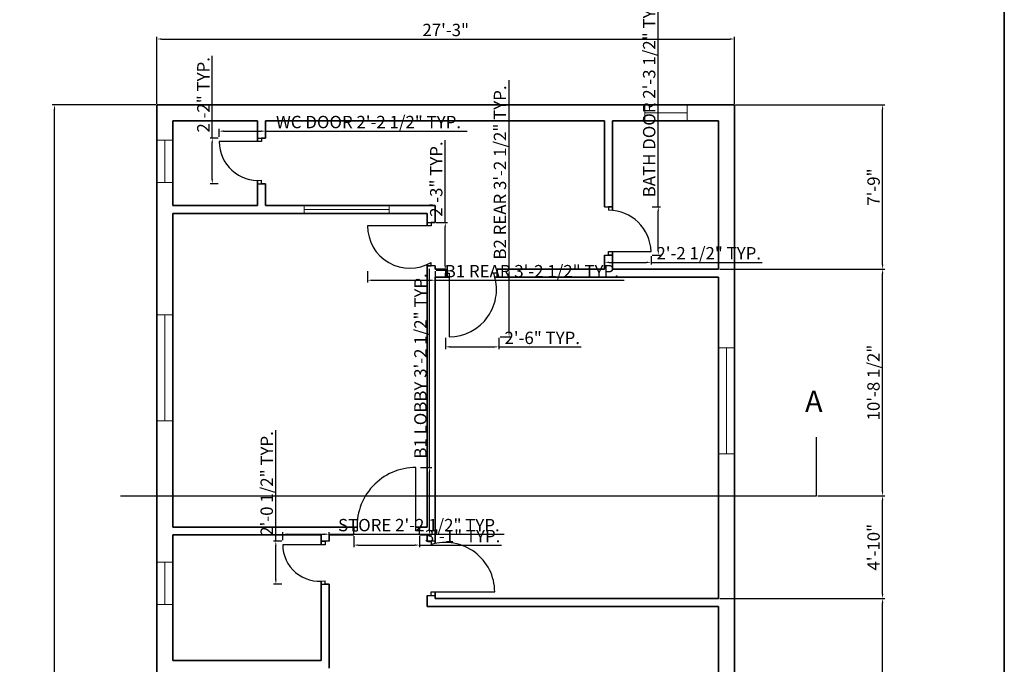
# Model space of a CAD drawing. Units: inches. Extents: x 1863 to 2938, y 1238 to 2492.
# Tile 11 of 12: x 2381 to 2938, y 1760 to 2125. Entities that reach past the tile are written whole.
import ezdxf

# ---------------------------------------------------------------- set-up
doc = ezdxf.new("R2010")
doc.units = ezdxf.units.IN
for name, color, linetype, lineweight in [('A-ANNO-DIMS', 2, 'Continuous', 18), ('A-ANNO-SYMB', 7, 'Continuous', 25), ('A-ANNO-TTLB', 7, 'Continuous', 35), ('A-DOOR', 3, 'Continuous', 25), ('A-GLAZ', 4, 'Continuous', 18), ('A-WALL', 7, 'Continuous', 35)]:
    doc.layers.add(name, color=color, linetype=linetype, lineweight=lineweight)
doc.styles.get("Standard").update_dxf_attribs({"font": 'arial.ttf'})
doc.dimstyles.new('ISO-25', dxfattribs={"dimtxt": 7, "dimasz": 2.5, "dimexe": 1.25, "dimexo": 0.625, "dimtad": 1, "dimdec": 0, "dimlunit": 3, "dimtxsty": 'Standard', "dimcen": 2.5, "dimadec": 0, "dimazin": 0, "dimtfac": 1, "dimtdec": 0, "dimtmove": 0, "dimatfit": 3, "dimfxl": 1, "dimarcsym": 0})

# ---------------------------------------------------------------- blocks, each defined once
blk = doc.blocks.new('DOOR-24-TOILET')
for p, q in [((24, 23.86), (0, 23.86)), ((21.75, 25.86), (26.25, 25.86)), ((26.25, 25.86), (24, 25.86)), ((24, 25.86), (24, 23.86)), ((21.75, 0), (26.25, 0)), ((24, 0), (24, 2)), ((26.25, 0), (24, 0))]:
    blk.add_line(p, q)
blk.add_arc((21.96, 23.86), 21.96, 180, 275.3383)
blk = doc.blocks.new('DOOR-36-BED1-REAR')
for p, q in [((36, 23.94), (0, 23.94)), ((33.75, 25.94), (38.25, 25.94)), ((38.25, 25.94), (36, 25.94)), ((36, 25.94), (36, 23.94)), ((38.25, 1.26), (33.75, 1.26)), ((33.75, 1.26), (36, 1.26)), ((36, 1.26), (36, 3.26))]:
    blk.add_line(p, q)
blk.add_arc((23.94, 23.94), 23.94, 180, 300.2375)
blk = doc.blocks.new('DOOR-24-BATH')
for p, q in [((0, 27.38), (4.5, 27.38)), ((4.5, 27.38), (2.25, 27.38)), ((2.25, 27.38), (2.25, 25.38)), ((0, 0), (4.5, 0)), ((2.25, 0), (2.25, 2)), ((2.25, 2), (26.25, 2)), ((4.5, 0), (2.25, 0))]:
    blk.add_line(p, q)
blk.add_arc((2.25, 1.37), 24.01, 1.5021, 90)
blk = doc.blocks.new('DOOR-36-BED2-REAR')
for p, q in [((0, 38.25), (0, 33.75)), ((0, 33.75), (0, 36)), ((0, 36), (2, 36)), ((2, 36), (2, 0)), ((29.25, 36), (27.25, 36)), ((29.25, 38.25), (29.25, 33.75)), ((29.25, 33.75), (29.25, 36))]:
    blk.add_line(p, q)
blk.add_arc((2, 26.86), 26.86, 270, 19.9084)
blk = doc.blocks.new('DOOR-36-BED2-LOBBY')
for p, q in [((0, 30.86), (4.5, 30.86)), ((2.25, 30.86), (2.25, 28.86)), ((0, 0), (4.5, 0)), ((2.25, 0), (2.25, 2)), ((2.25, 2), (38.25, 2))]:
    blk.add_line(p, q)
blk.add_arc((10.23, 2), 28.02, 0, 106.5507)
blk = doc.blocks.new('DOOR-24-STORE')
for p, q in [((24, 22.39), (0, 22.39)), ((26.25, 24.39), (21.75, 24.39)), ((21.75, 24.39), (24, 24.39)), ((24, 24.39), (24, 22.39)), ((24, 0), (24, 2)), ((21.75, 0), (26.25, 0)), ((26.25, 0), (24, 0))]:
    blk.add_line(p, q)
blk.add_arc((20.66, 22.39), 20.66, 180, 279.3111)
blk = doc.blocks.new('DOOR-36-BED1-LOBBY')
for p, q in [((35.21, 2.25), (35.21, 38.25)), ((0, 0), (0, 4.5)), ((0, 4.5), (0, 2.25)), ((0, 2.25), (2, 2.25)), ((37.21, 2.25), (35.21, 2.25)), ((37.21, 0), (37.21, 4.5)), ((37.21, 4.5), (37.21, 2.25))]:
    blk.add_line(p, q)
blk.add_arc((35.21, 4.93), 33.32, 90, 184.6101)
blk = doc.blocks.new('WIN-24')
for p, q in [((0, 24), (9, 24)), ((9, 24), (4.5, 24)), ((4.5, 24), (4.5, 0)), ((4.5, 0), (0, 0)), ((0, 0), (9, 0))]:
    blk.add_line(p, q)
blk = doc.blocks.new('WIN-48')
for p, q in [((0, 4.5), (0, 0)), ((0, 0), (0, 2.25)), ((0, 2.25), (48, 2.25)), ((48, 2.25), (48, 4.5)), ((48, 4.5), (48, 0))]:
    blk.add_line(p, q)
blk = doc.blocks.new('WIN-60')
for p, q in [((0, 60), (9, 60)), ((9, 60), (4.5, 60)), ((4.5, 60), (4.5, 0)), ((4.5, 0), (0, 0)), ((0, 0), (9, 0))]:
    blk.add_line(p, q)
blk = doc.blocks.new('WIN-24-STORE')
for p, q in [((0, 24), (9, 24)), ((9, 24), (4.5, 24)), ((4.5, 24), (4.5, 0)), ((9, 0), (0, 0)), ((4.5, 0), (9, 0))]:
    blk.add_line(p, q)
blk = doc.blocks.new('*D40')
at = {"layer": 'A-ANNO-DIMS', "color": 0, "lineweight": -2, "transparency": 16777216}
for p, q in [((2493.88, 2058.42), (2493.88, 2062.98)), ((2520.13, 2058.42), (2520.13, 2062.98)), ((2496.38, 2061.73), (2517.63, 2061.73)), ((2520.13, 2061.73), (2634.21, 2061.73))]:
    blk.add_line(p, q, dxfattribs=at)
at = {"layer": 'A-ANNO-DIMS', "color": 0, "transparency": 16777216}
for points in [[(2496.38, 2062.15), (2496.38, 2061.31), (2493.88, 2061.73)], [(2517.63, 2062.15), (2517.63, 2061.31), (2520.13, 2061.73)]]:
    blk.add_solid(points, dxfattribs=at)
at = {"layer": 'Defpoints', "color": 0, "transparency": 16777216}
for p in [(2493.88, 2057.79), (2520.13, 2061.73), (2520.13, 2057.79)]:
    blk.add_point(p, dxfattribs=at)
at = {"layer": 'A-ANNO-DIMS', "color": 0, "transparency": 16777216, "insert": (2578.42, 2065.98), "char_height": 7, "attachment_point": 5}
blk.add_mtext('WC DOOR 2\'-2 1/2" TYP.', dxfattribs=at)
blk = doc.blocks.new('*D41')
at = {"layer": 'A-ANNO-DIMS', "color": 0, "lineweight": -2, "transparency": 16777216}
for p, q in [((2489.94, 2057.79), (2489.94, 2104.33)), ((2493.26, 2057.79), (2488.69, 2057.79)), ((2489.94, 2034.43), (2489.94, 2055.29)), ((2493.26, 2031.93), (2488.69, 2031.93))]:
    blk.add_line(p, q, dxfattribs=at)
at = {"layer": 'A-ANNO-DIMS', "color": 0, "transparency": 16777216}
for points in [[(2489.53, 2055.29), (2490.36, 2055.29), (2489.94, 2057.79)], [(2489.53, 2034.43), (2490.36, 2034.43), (2489.94, 2031.93)]]:
    blk.add_solid(points, dxfattribs=at)
at = {"layer": 'Defpoints', "color": 0, "transparency": 16777216}
for p in [(2489.94, 2057.79), (2493.88, 2057.79), (2493.88, 2031.93)]:
    blk.add_point(p, dxfattribs=at)
at = {"layer": 'A-ANNO-DIMS', "color": 0, "transparency": 16777216, "insert": (2485.8, 2082.31), "char_height": 7, "attachment_point": 5, "rotation": 90}
blk.add_mtext('2\'-2" TYP.', dxfattribs=at)
blk = doc.blocks.new('*D42')
at = {"layer": 'A-ANNO-DIMS', "color": 0, "lineweight": -2, "transparency": 16777216}
for p, q in [((2577.88, 1982.4), (2577.88, 1976.04)), ((2616.13, 1982.4), (2616.13, 1976.04)), ((2580.38, 1977.29), (2613.63, 1977.29)), ((2616.13, 1977.29), (2723.11, 1977.29))]:
    blk.add_line(p, q, dxfattribs=at)
at = {"layer": 'A-ANNO-DIMS', "color": 0, "transparency": 16777216}
for points in [[(2580.38, 1977.7), (2580.38, 1976.87), (2577.88, 1977.29)], [(2613.63, 1977.7), (2613.63, 1976.87), (2616.13, 1977.29)]]:
    blk.add_solid(points, dxfattribs=at)
at = {"layer": 'Defpoints', "color": 0, "transparency": 16777216}
for p in [(2577.88, 1983.02), (2616.13, 1983.02), (2616.13, 1977.29)]:
    blk.add_point(p, dxfattribs=at)
at = {"layer": 'A-ANNO-DIMS', "color": 0, "transparency": 16777216, "insert": (2670.87, 1981.53), "char_height": 7, "attachment_point": 5}
blk.add_mtext('B1 REAR 3\'-2 1/2" TYP.', dxfattribs=at)
blk = doc.blocks.new('*D43')
at = {"layer": 'A-ANNO-DIMS', "color": 0, "lineweight": -2, "transparency": 16777216}
for p, q in [((2621.87, 2010.05), (2621.87, 2056.59)), ((2616.76, 2010.05), (2623.12, 2010.05)), ((2621.87, 1985.52), (2621.87, 2007.55)), ((2616.76, 1983.02), (2623.12, 1983.02))]:
    blk.add_line(p, q, dxfattribs=at)
at = {"layer": 'A-ANNO-DIMS', "color": 0, "transparency": 16777216}
for points in [[(2621.45, 2007.55), (2622.29, 2007.55), (2621.87, 2010.05)], [(2621.45, 1985.52), (2622.29, 1985.52), (2621.87, 1983.02)]]:
    blk.add_solid(points, dxfattribs=at)
at = {"layer": 'Defpoints', "color": 0, "transparency": 16777216}
for p in [(2616.13, 2010.05), (2621.87, 2010.05), (2616.13, 1983.02)]:
    blk.add_point(p, dxfattribs=at)
at = {"layer": 'A-ANNO-DIMS', "color": 0, "transparency": 16777216, "insert": (2617.67, 2034.57), "char_height": 7, "attachment_point": 5, "rotation": 90}
blk.add_mtext('2\'-3" TYP.', dxfattribs=at)
blk = doc.blocks.new('*D44')
at = {"layer": 'A-ANNO-DIMS', "color": 0, "lineweight": -2, "transparency": 16777216}
for p, q in [((2742.49, 2018.92), (2742.49, 2142.19)), ((2739.01, 2018.92), (2743.74, 2018.92)), ((2742.49, 1994.04), (2742.49, 2016.42)), ((2739.01, 1991.54), (2743.74, 1991.54))]:
    blk.add_line(p, q, dxfattribs=at)
at = {"layer": 'A-ANNO-DIMS', "color": 0, "transparency": 16777216}
for points in [[(2742.07, 2016.42), (2742.91, 2016.42), (2742.49, 2018.92)], [(2742.07, 1994.04), (2742.91, 1994.04), (2742.49, 1991.54)]]:
    blk.add_solid(points, dxfattribs=at)
at = {"layer": 'Defpoints', "color": 0, "transparency": 16777216}
for p in [(2738.38, 2018.92), (2742.49, 2018.92), (2738.38, 1991.54)]:
    blk.add_point(p, dxfattribs=at)
at = {"layer": 'A-ANNO-DIMS', "color": 0, "transparency": 16777216, "insert": (2738.24, 2081.8), "char_height": 7, "attachment_point": 5, "rotation": 90}
blk.add_mtext('BATH DOOR 2\'-3 1/2" TYP.', dxfattribs=at)
blk = doc.blocks.new('*D45')
at = {"layer": 'A-ANNO-DIMS', "color": 0, "lineweight": -2, "transparency": 16777216}
for p, q in [((2712.13, 1990.91), (2712.13, 1986.18)), ((2738.38, 1990.91), (2738.38, 1986.18)), ((2714.63, 1987.43), (2735.88, 1987.43)), ((2738.38, 1987.43), (2801.23, 1987.43))]:
    blk.add_line(p, q, dxfattribs=at)
at = {"layer": 'A-ANNO-DIMS', "color": 0, "transparency": 16777216}
for points in [[(2714.63, 1987.85), (2714.63, 1987.01), (2712.13, 1987.43)], [(2735.88, 1987.85), (2735.88, 1987.01), (2738.38, 1987.43)]]:
    blk.add_solid(points, dxfattribs=at)
at = {"layer": 'Defpoints', "color": 0, "transparency": 16777216}
for p in [(2712.13, 1991.54), (2738.38, 1991.54), (2738.38, 1987.43)]:
    blk.add_point(p, dxfattribs=at)
at = {"layer": 'A-ANNO-DIMS', "color": 0, "transparency": 16777216, "insert": (2771.06, 1991.68), "char_height": 7, "attachment_point": 5}
blk.add_mtext('2\'-2 1/2" TYP.', dxfattribs=at)
blk = doc.blocks.new('*D46')
at = {"layer": 'A-ANNO-DIMS', "color": 0, "lineweight": -2, "transparency": 16777216}
for p, q in [((2658.01, 1983.56), (2658.01, 2090.55)), ((2652.89, 1983.56), (2659.26, 1983.56)), ((2658.01, 1947.81), (2658.01, 1981.06)), ((2652.89, 1945.31), (2659.26, 1945.31))]:
    blk.add_line(p, q, dxfattribs=at)
at = {"layer": 'A-ANNO-DIMS', "color": 0, "transparency": 16777216}
for points in [[(2657.59, 1981.06), (2658.42, 1981.06), (2658.01, 1983.56)], [(2657.59, 1947.81), (2658.42, 1947.81), (2658.01, 1945.31)]]:
    blk.add_solid(points, dxfattribs=at)
at = {"layer": 'Defpoints', "color": 0, "transparency": 16777216}
for p in [(2652.27, 1983.56), (2658.01, 1983.56), (2652.27, 1945.31)]:
    blk.add_point(p, dxfattribs=at)
at = {"layer": 'A-ANNO-DIMS', "color": 0, "transparency": 16777216, "insert": (2653.76, 2038.3), "char_height": 7, "attachment_point": 5, "rotation": 90}
blk.add_mtext('B2 REAR 3\'-2 1/2" TYP.', dxfattribs=at)
blk = doc.blocks.new('*D47')
at = {"layer": 'A-ANNO-DIMS', "color": 0, "lineweight": -2, "transparency": 16777216}
for p, q in [((2622.04, 1944.69), (2622.04, 1938.32)), ((2652.27, 1944.69), (2652.27, 1938.32)), ((2624.54, 1939.57), (2649.77, 1939.57)), ((2652.27, 1939.57), (2698.81, 1939.57))]:
    blk.add_line(p, q, dxfattribs=at)
at = {"layer": 'A-ANNO-DIMS', "color": 0, "transparency": 16777216}
for points in [[(2624.54, 1939.99), (2624.54, 1939.16), (2622.04, 1939.57)], [(2649.77, 1939.99), (2649.77, 1939.16), (2652.27, 1939.57)]]:
    blk.add_solid(points, dxfattribs=at)
at = {"layer": 'Defpoints', "color": 0, "transparency": 16777216}
for p in [(2622.04, 1945.31), (2652.27, 1945.31), (2652.27, 1939.57)]:
    blk.add_point(p, dxfattribs=at)
at = {"layer": 'A-ANNO-DIMS', "color": 0, "transparency": 16777216, "insert": (2676.79, 1943.77), "char_height": 7, "attachment_point": 5}
blk.add_mtext('2\'-6" TYP.', dxfattribs=at)
blk = doc.blocks.new('*D50')
at = {"layer": 'A-ANNO-DIMS', "color": 0, "lineweight": -2, "transparency": 16777216}
for p, q in [((2529.88, 1830.17), (2529.88, 1834.73)), ((2556.13, 1830.17), (2556.13, 1834.73)), ((2532.38, 1833.48), (2553.63, 1833.48)), ((2556.13, 1833.48), (2655.23, 1833.48))]:
    blk.add_line(p, q, dxfattribs=at)
at = {"layer": 'A-ANNO-DIMS', "color": 0, "transparency": 16777216}
for points in [[(2532.38, 1833.9), (2532.38, 1833.06), (2529.88, 1833.48)], [(2553.63, 1833.9), (2553.63, 1833.06), (2556.13, 1833.48)]]:
    blk.add_solid(points, dxfattribs=at)
at = {"layer": 'Defpoints', "color": 0, "transparency": 16777216}
for p in [(2529.88, 1829.54), (2556.13, 1833.48), (2556.13, 1829.54)]:
    blk.add_point(p, dxfattribs=at)
at = {"layer": 'A-ANNO-DIMS', "color": 0, "transparency": 16777216, "insert": (2606.93, 1837.73), "char_height": 7, "attachment_point": 5}
blk.add_mtext('STORE 2\'-2 1/2" TYP.', dxfattribs=at)
blk = doc.blocks.new('*D51')
at = {"layer": 'A-ANNO-DIMS', "color": 0, "lineweight": -2, "transparency": 16777216}
for p, q in [((2525.94, 1829.54), (2525.94, 1892.39)), ((2529.26, 1829.54), (2524.69, 1829.54)), ((2525.94, 1807.66), (2525.94, 1827.04)), ((2529.26, 1805.16), (2524.69, 1805.16))]:
    blk.add_line(p, q, dxfattribs=at)
at = {"layer": 'A-ANNO-DIMS', "color": 0, "transparency": 16777216}
for points in [[(2525.53, 1827.04), (2526.36, 1827.04), (2525.94, 1829.54)], [(2525.53, 1807.66), (2526.36, 1807.66), (2525.94, 1805.16)]]:
    blk.add_solid(points, dxfattribs=at)
at = {"layer": 'Defpoints', "color": 0, "transparency": 16777216}
for p in [(2525.94, 1829.54), (2529.88, 1829.54), (2529.88, 1805.16)]:
    blk.add_point(p, dxfattribs=at)
at = {"layer": 'A-ANNO-DIMS', "color": 0, "transparency": 16777216, "insert": (2521.7, 1862.22), "char_height": 7, "attachment_point": 5, "rotation": 90}
blk.add_mtext('2\'-0 1/2" TYP.', dxfattribs=at)
blk = doc.blocks.new('*D52')
at = {"layer": 'A-ANNO-DIMS', "color": 0, "lineweight": -2, "transparency": 16777216}
for p, q in [((2612.98, 1871.31), (2612.98, 1983.74)), ((2607.87, 1871.31), (2614.23, 1871.31)), ((2612.98, 1835.56), (2612.98, 1868.81)), ((2607.87, 1833.06), (2614.23, 1833.06))]:
    blk.add_line(p, q, dxfattribs=at)
at = {"layer": 'A-ANNO-DIMS', "color": 0, "transparency": 16777216}
for points in [[(2612.56, 1868.81), (2613.4, 1868.81), (2612.98, 1871.31)], [(2612.56, 1835.56), (2613.4, 1835.56), (2612.98, 1833.06)]]:
    blk.add_solid(points, dxfattribs=at)
at = {"layer": 'Defpoints', "color": 0, "transparency": 16777216}
for p in [(2607.24, 1871.31), (2612.98, 1871.31), (2607.24, 1833.06)]:
    blk.add_point(p, dxfattribs=at)
at = {"layer": 'A-ANNO-DIMS', "color": 0, "transparency": 16777216, "insert": (2608.73, 1928.78), "char_height": 7, "attachment_point": 5, "rotation": 90}
blk.add_mtext('B1 LOBBY 3\'-2 1/2" TYP.', dxfattribs=at)
blk = doc.blocks.new('*D53')
at = {"layer": 'A-ANNO-DIMS', "color": 0, "lineweight": -2, "transparency": 16777216}
for p, q in [((2570.03, 1832.44), (2570.03, 1826.07)), ((2607.24, 1832.44), (2607.24, 1826.07)), ((2572.53, 1827.32), (2604.74, 1827.32)), ((2607.24, 1827.32), (2653.66, 1827.32))]:
    blk.add_line(p, q, dxfattribs=at)
at = {"layer": 'A-ANNO-DIMS', "color": 0, "transparency": 16777216}
for points in [[(2572.53, 1827.74), (2572.53, 1826.91), (2570.03, 1827.32)], [(2604.74, 1827.74), (2604.74, 1826.91), (2607.24, 1827.32)]]:
    blk.add_solid(points, dxfattribs=at)
at = {"layer": 'Defpoints', "color": 0, "transparency": 16777216}
for p in [(2570.03, 1833.06), (2607.24, 1833.06), (2607.24, 1827.32)]:
    blk.add_point(p, dxfattribs=at)
at = {"layer": 'A-ANNO-DIMS', "color": 0, "transparency": 16777216, "insert": (2631.7, 1831.53), "char_height": 7, "attachment_point": 5}
blk.add_mtext('3\'-1" TYP.', dxfattribs=at)
blk = doc.blocks.new('*D64')
at = {"layer": 'A-ANNO-DIMS', "color": 0, "lineweight": -2, "transparency": 16777216}
for p, q in [((2458.63, 2077.19), (2458.63, 2115.16)), ((2461.13, 2113.91), (2783.13, 2113.91)), ((2785.63, 2077.19), (2785.63, 2115.16))]:
    blk.add_line(p, q, dxfattribs=at)
at = {"layer": 'A-ANNO-DIMS', "color": 0, "transparency": 16777216}
for points in [[(2461.13, 2114.33), (2461.13, 2113.5), (2458.63, 2113.91)], [(2783.13, 2114.33), (2783.13, 2113.5), (2785.63, 2113.91)]]:
    blk.add_solid(points, dxfattribs=at)
at = {"layer": 'Defpoints', "color": 0, "transparency": 16777216}
for p in [(2785.63, 2113.91), (2458.63, 2076.56), (2785.63, 2076.56)]:
    blk.add_point(p, dxfattribs=at)
at = {"layer": 'A-ANNO-DIMS', "color": 0, "transparency": 16777216, "insert": (2622.13, 2118.11), "char_height": 7, "attachment_point": 5}
blk.add_mtext('27\'-3"', dxfattribs=at)
blk = doc.blocks.new('*D65')
at = {"layer": 'A-ANNO-DIMS', "color": 0, "lineweight": -2, "transparency": 16777216}
for p, q in [((2458.01, 2076.56), (2399.39, 2076.56)), ((2400.64, 1342.06), (2400.64, 2074.06)), ((2458.01, 1339.56), (2399.39, 1339.56))]:
    blk.add_line(p, q, dxfattribs=at)
at = {"layer": 'A-ANNO-DIMS', "color": 0, "transparency": 16777216}
for points in [[(2400.22, 2074.06), (2401.06, 2074.06), (2400.64, 2076.56)], [(2400.22, 1342.06), (2401.06, 1342.06), (2400.64, 1339.56)]]:
    blk.add_solid(points, dxfattribs=at)
at = {"layer": 'Defpoints', "color": 0, "transparency": 16777216}
for p in [(2400.64, 2076.56), (2458.63, 2076.56), (2458.63, 1339.56)]:
    blk.add_point(p, dxfattribs=at)
at = {"layer": 'A-ANNO-DIMS', "color": 0, "transparency": 16777216, "insert": (2396.44, 1708.06), "char_height": 7, "attachment_point": 5, "rotation": 90}
blk.add_mtext('61\'-5"', dxfattribs=at)
blk = doc.blocks.new('*D67')
at = {"layer": 'A-ANNO-DIMS', "color": 0, "lineweight": -2, "transparency": 16777216}
for p, q in [((2777.26, 1797.06), (2870.74, 1797.06)), ((2869.49, 1579.06), (2869.49, 1794.56)), ((2777.26, 1576.56), (2870.74, 1576.56))]:
    blk.add_line(p, q, dxfattribs=at)
at = {"layer": 'A-ANNO-DIMS', "color": 0, "transparency": 16777216}
for points in [[(2869.07, 1794.56), (2869.91, 1794.56), (2869.49, 1797.06)], [(2869.07, 1579.06), (2869.91, 1579.06), (2869.49, 1576.56)]]:
    blk.add_solid(points, dxfattribs=at)
at = {"layer": 'Defpoints', "color": 0, "transparency": 16777216}
for p in [(2776.63, 1797.06), (2869.49, 1797.06), (2776.63, 1576.56)]:
    blk.add_point(p, dxfattribs=at)
at = {"layer": 'A-ANNO-DIMS', "color": 0, "transparency": 16777216, "insert": (2865.25, 1686.81), "char_height": 7, "attachment_point": 5, "rotation": 90}
blk.add_mtext('18\'-4 1/2"', dxfattribs=at)
blk = doc.blocks.new('*D68')
at = {"layer": 'A-ANNO-DIMS', "color": 0, "lineweight": -2, "transparency": 16777216}
for p, q in [((2832.77, 1855.17), (2870.74, 1855.17)), ((2869.49, 1799.56), (2869.49, 1852.67)), ((2777.26, 1797.06), (2870.74, 1797.06))]:
    blk.add_line(p, q, dxfattribs=at)
at = {"layer": 'A-ANNO-DIMS', "color": 0, "transparency": 16777216}
for points in [[(2869.07, 1852.67), (2869.91, 1852.67), (2869.49, 1855.17)], [(2869.07, 1799.56), (2869.91, 1799.56), (2869.49, 1797.06)]]:
    blk.add_solid(points, dxfattribs=at)
at = {"layer": 'Defpoints', "color": 0, "transparency": 16777216}
for p in [(2832.14, 1855.17), (2869.49, 1855.17), (2776.63, 1797.06)]:
    blk.add_point(p, dxfattribs=at)
at = {"layer": 'A-ANNO-DIMS', "color": 0, "transparency": 16777216, "insert": (2865.29, 1826.12), "char_height": 7, "attachment_point": 5, "rotation": 90}
blk.add_mtext('4\'-10"', dxfattribs=at)
blk = doc.blocks.new('*D69')
at = {"layer": 'A-ANNO-DIMS', "color": 0, "lineweight": -2, "transparency": 16777216}
for p, q in [((2777.26, 1983.56), (2870.74, 1983.56)), ((2869.49, 1857.67), (2869.49, 1981.06)), ((2832.77, 1855.17), (2870.74, 1855.17))]:
    blk.add_line(p, q, dxfattribs=at)
at = {"layer": 'A-ANNO-DIMS', "color": 0, "transparency": 16777216}
for points in [[(2869.07, 1981.06), (2869.91, 1981.06), (2869.49, 1983.56)], [(2869.07, 1857.67), (2869.91, 1857.67), (2869.49, 1855.17)]]:
    blk.add_solid(points, dxfattribs=at)
at = {"layer": 'Defpoints', "color": 0, "transparency": 16777216}
for p in [(2776.63, 1983.56), (2869.49, 1983.56), (2832.14, 1855.17)]:
    blk.add_point(p, dxfattribs=at)
at = {"layer": 'A-ANNO-DIMS', "color": 0, "transparency": 16777216, "insert": (2865.25, 1919.37), "char_height": 7, "attachment_point": 5, "rotation": 90}
blk.add_mtext('10\'-8 1/2"', dxfattribs=at)
blk = doc.blocks.new('*D70')
at = {"layer": 'A-ANNO-DIMS', "color": 0, "lineweight": -2, "transparency": 16777216}
for p, q in [((2786.26, 2076.56), (2870.74, 2076.56)), ((2869.49, 1986.06), (2869.49, 2074.06)), ((2777.26, 1983.56), (2870.74, 1983.56))]:
    blk.add_line(p, q, dxfattribs=at)
at = {"layer": 'A-ANNO-DIMS', "color": 0, "transparency": 16777216}
for points in [[(2869.07, 2074.06), (2869.91, 2074.06), (2869.49, 2076.56)], [(2869.07, 1986.06), (2869.91, 1986.06), (2869.49, 1983.56)]]:
    blk.add_solid(points, dxfattribs=at)
at = {"layer": 'Defpoints', "color": 0, "transparency": 16777216}
for p in [(2785.63, 2076.56), (2869.49, 2076.56), (2776.63, 1983.56)]:
    blk.add_point(p, dxfattribs=at)
at = {"layer": 'A-ANNO-DIMS', "color": 0, "transparency": 16777216, "insert": (2865.29, 2030.06), "char_height": 7, "attachment_point": 5, "rotation": 90}
blk.add_mtext('7\'-9"', dxfattribs=at)

msp = doc.modelspace()

# ---------------------------------------------------------------- linework, layer by layer
at = {"layer": 'A-ANNO-SYMB'}
for p, q in [((2832.14, 1855.17), (2832.14, 1888.53)), ((2437.99, 1855.17), (2832.14, 1855.17))]:
    msp.add_line(p, q, dxfattribs=at)
at = {"layer": 'A-ANNO-TTLB'}
msp.add_lwpolyline([(1863.2, 2492.19), (2938.41, 2492.19), (2938.41, 1253.47), (1863.2, 1253.47)], close=True, dxfattribs=at)
at = {"layer": 'A-WALL'}
for p, q in [((2458.63, 2076.56), (2458.63, 1339.56)), ((2458.63, 2076.56), (2458.63, 1339.56)), ((2458.63, 2076.56), (2785.63, 2076.56)), ((2785.63, 2076.56), (2785.63, 1495.56)), ((2467.63, 2067.56), (2467.63, 2019.56)), ((2467.63, 2067.56), (2515.63, 2067.56)), ((2515.63, 2067.56), (2515.63, 2055.79)), ((2520.13, 2067.56), (2520.13, 2057.79)), ((2520.13, 2067.56), (2712.13, 2067.56)), ((2712.13, 2067.56), (2712.13, 2018.92)), ((2716.63, 2067.56), (2716.63, 2016.81)), ((2716.63, 2067.56), (2776.63, 2067.56)), ((2776.63, 2067.56), (2776.63, 1983.56)), ((2515.63, 2033.84), (2515.63, 2019.56)), ((2520.13, 2031.93), (2520.13, 2019.56)), ((2467.63, 2019.56), (2515.63, 2019.56)), ((2520.13, 2019.56), (2616.13, 2019.56)), ((2616.13, 2019.56), (2616.13, 2010.05)), ((2467.63, 2015.06), (2467.63, 1837.56)), ((2467.63, 2015.06), (2611.63, 2015.06)), ((2611.63, 2015.06), (2611.63, 2008.05)), ((2712.13, 1991.54), (2712.13, 1983.56)), ((2716.63, 1993.54), (2716.63, 1983.56)), ((2611.63, 1986.21), (2611.63, 1837.56)), ((2616.13, 1985.37), (2616.13, 1983.56)), ((2616.13, 1983.56), (2622.04, 1983.56)), ((2651.29, 1983.56), (2712.13, 1983.56)), ((2716.63, 1983.56), (2776.63, 1983.56)), ((2616.13, 1979.06), (2616.13, 1828.23)), ((2616.13, 1979.06), (2624.04, 1979.06)), ((2649.99, 1979.06), (2776.63, 1979.06)), ((2776.63, 1979.06), (2776.63, 1797.06)), ((2467.63, 1837.56), (2570.03, 1837.56)), ((2556.13, 1837.56), (2571.92, 1837.56)), ((2605.24, 1837.56), (2611.63, 1837.56)), ((2467.63, 1833.06), (2467.63, 1762.06)), ((2467.63, 1833.06), (2551.63, 1833.06)), ((2551.63, 1833.06), (2551.63, 1827.54)), ((2551.63, 1833.06), (2551.63, 1827.54)), ((2556.13, 1833.06), (2556.13, 1829.54)), ((2556.13, 1833.06), (2556.13, 1829.54)), ((2556.13, 1833.06), (2570.03, 1833.06)), ((2607.24, 1833.06), (2611.63, 1833.06)), ((2611.63, 1833.06), (2611.63, 1829.66)), ((2551.63, 1806.91), (2551.63, 1762.06)), ((2551.63, 1806.91), (2551.63, 1762.06)), ((2556.13, 1805.16), (2556.13, 1762.06)), ((2556.13, 1805.16), (2556.13, 1762.06)), ((2616.13, 1800.8), (2616.13, 1797.06)), ((2611.63, 1798.8), (2611.63, 1792.56)), ((2616.13, 1797.06), (2776.63, 1797.06)), ((2616.13, 1792.56), (2611.63, 1792.56)), ((2616.13, 1792.56), (2776.63, 1792.56)), ((2776.63, 1792.56), (2776.63, 1576.56)), ((2467.63, 1762.06), (2551.63, 1762.06)), ((2556.13, 1762.06), (2556.13, 1757.56))]:
    msp.add_line(p, q, dxfattribs=at)

# ---------------------------------------------------------------- block references
at = {"layer": 'A-DOOR'}
for name, p in [('DOOR-24-TOILET', (2493.88, 2031.93)), ('DOOR-24-BATH', (2712.13, 1991.54)), ('DOOR-36-BED1-REAR', (2577.88, 1984.11)), ('DOOR-36-BED2-REAR', (2622.04, 1945.31)), ('DOOR-36-BED1-LOBBY', (2570.03, 1833.06)), ('DOOR-24-STORE', (2529.88, 1805.16)), ('DOOR-36-BED2-LOBBY', (2611.63, 1798.8))]:
    msp.add_blockref(name, p, dxfattribs=at)
at = {"layer": 'A-GLAZ'}
for p, rotation in [((2734.89, 2076.56), 270.0000000000037), ((2467.63, 2056.59), 180)]:
    msp.add_blockref('WIN-24', p, dxfattribs=dict(at, rotation=rotation))
for name, p in [('WIN-48', (2542.04, 2015.06)), ('WIN-60', (2458.63, 1897.7)), ('WIN-60', (2776.63, 1879.02)), ('WIN-24-STORE', (2458.63, 1793.66))]:
    msp.add_blockref(name, p, dxfattribs=at)

# ---------------------------------------------------------------- texts
at = {"layer": 'A-ANNO-SYMB', "insert": (2825.58, 1914.74), "char_height": 12, "attachment_point": 1}
msp.add_mtext_dynamic_manual_height_columns('A', width=32.5779, gutter_width=12.5, heights=[0], dxfattribs=at)

# ---------------------------------------------------------------- dimensions: what is measured, and where the dimension line sits
at = {"layer": 'A-ANNO-DIMS'}
for base, p1, p2, text, picture, middle in [((2742.49, 2018.92), (2738.38, 1991.54), (2738.38, 2018.92), 'BATH DOOR <> TYP.', '*D44', (2738.24, 2081.8)), ((2489.94, 2057.79), (2493.88, 2031.93), (2493.88, 2057.79), '<> TYP.', '*D41', (2485.8, 2082.31)), ((2658.00554332, 1983.5618837), (2652.26804332, 1945.3118837), (2652.26804332, 1983.5618837), 'B2 REAR <> TYP.', '*D46', (2653.75878343, 2038.30352763)), ((2621.87, 2010.05), (2616.13, 1983.02), (2616.13, 2010.05), '<> TYP.', '*D43', (2617.67, 2034.57)), ((2612.9791649, 1871.3118837), (2607.2416649, 1833.0618837), (2607.2416649, 1871.3118837), 'B1 LOBBY <> TYP.', '*D52', (2608.73001756, 1928.7752193)), ((2525.94, 1829.54), (2529.88, 1805.16), (2529.88, 1829.54), '<> TYP.', '*D51', (2521.7, 1862.22))]:
    dim = msp.add_linear_dim(base=base, p1=p1, p2=p2, angle=90, text=text, dimstyle='ISO-25', override={"dimdec": 1, "dimlfac": 1, "dimrnd": 0, "dimzin": 1, "dimdsep": 46, "dimlunit": 4, "dimfrac": 2}, dxfattribs=at)
    dim.commit()
    dim.dimension.update_dxf_attribs({"geometry": picture, "text_midpoint": middle})
dim = msp.add_linear_dim(base=(2785.63, 2113.91), p1=(2458.63, 2076.56), p2=(2785.63, 2076.56), dimstyle='ISO-25', override={"dimdec": 1, "dimlfac": 1, "dimrnd": 0, "dimzin": 1, "dimdsep": 46, "dimlunit": 4, "dimfrac": 2}, dxfattribs=at)
dim.commit()
dim.dimension.update_dxf_attribs({"geometry": '*D64', "text_midpoint": (2622.13, 2118.11)})
for base, p1, p2, text, picture, middle in [((2520.13159295, 2061.73098911), (2493.88159295, 2057.79348911), (2520.13159295, 2057.79348911), 'WC DOOR <> TYP.', '*D40', (2578.42098586, 2065.977749)), ((2616.13159295, 1977.28715324), (2577.88159295, 1983.02465324), (2616.13159295, 1983.02465324), 'B1 REAR <> TYP.', '*D42', (2670.87323688, 1981.53391313)), ((2738.38159295, 1987.43111512), (2712.13159295, 1991.53794883), (2738.38159295, 1991.53794883), '<> TYP.', '*D45', (2771.05604725, 1991.67548756)), ((2652.27, 1939.57), (2622.04, 1945.31), (2652.27, 1945.31), '<> TYP.', '*D47', (2676.79, 1943.77)), ((2556.13159295, 1833.48025876), (2529.88159295, 1829.54275876), (2556.13159295, 1829.54275876), 'STORE <> TYP.', '*D50', (2606.93155885, 1837.72701865)), ((2607.24, 1827.32), (2570.03, 1833.06), (2607.24, 1833.06), '<> TYP.', '*D53', (2631.7, 1831.53))]:
    dim = msp.add_linear_dim(base=base, p1=p1, p2=p2, text=text, dimstyle='ISO-25', override={"dimdec": 1, "dimlfac": 1, "dimrnd": 0, "dimzin": 1, "dimdsep": 46, "dimlunit": 4, "dimfrac": 2}, dxfattribs=at)
    dim.commit()
    dim.dimension.update_dxf_attribs({"geometry": picture, "text_midpoint": middle})
for base, p1, p2, picture, middle in [((2400.64, 2076.56), (2458.63, 1339.56), (2458.63, 2076.56), '*D65', (2396.44, 1708.06)), ((2869.49, 2076.56), (2776.63, 1983.56), (2785.63, 2076.56), '*D70', (2865.29, 2030.06)), ((2869.49, 1983.56), (2832.14, 1855.17), (2776.63, 1983.56), '*D69', (2865.25, 1919.37)), ((2869.49, 1855.17), (2776.63, 1797.06), (2832.14, 1855.17), '*D68', (2865.29, 1826.12)), ((2869.49, 1797.06), (2776.63, 1576.56), (2776.63, 1797.06), '*D67', (2865.25, 1686.81))]:
    dim = msp.add_linear_dim(base=base, p1=p1, p2=p2, angle=90, dimstyle='ISO-25', override={"dimdec": 1, "dimlfac": 1, "dimrnd": 0, "dimzin": 1, "dimdsep": 46, "dimlunit": 4, "dimfrac": 2}, dxfattribs=at)
    dim.commit()
    dim.dimension.update_dxf_attribs({"geometry": picture, "text_midpoint": middle})

doc.saveas('drawing.dxf')
